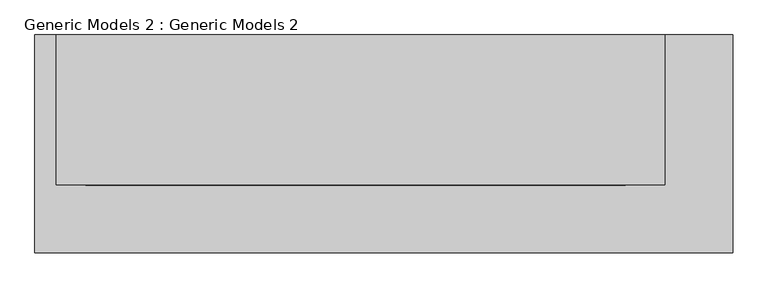
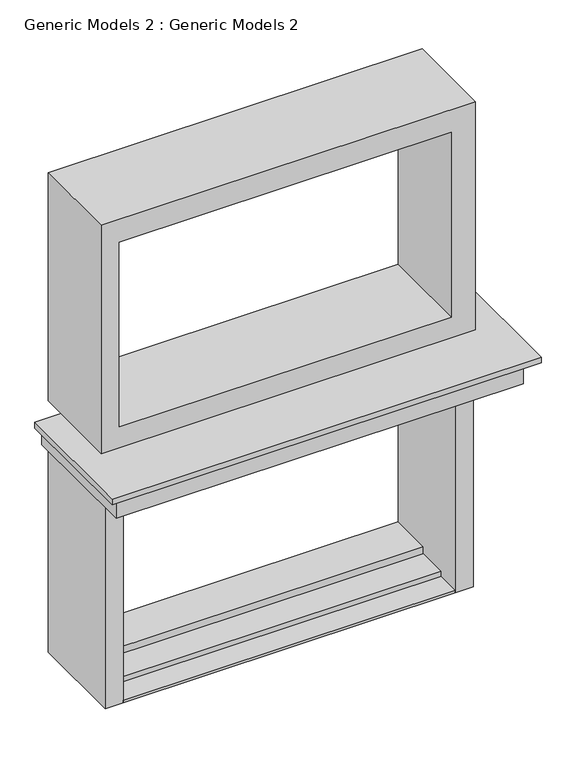
"""IFC4 building model written with IfcOpenShell, lengths in millimetres: proxy geometry, Generic Models 2 : Generic Models 2."""

from ifc_helpers import new_model, si_unit, frame, origin, origin_with_axes, place, context, project, spatial, polyline, outline, extrude, source, transform, mapped, element, save


def generic_models_2_generic_models_2_d251e182(model_context):
    return source(origin(), model_context, "Body", "SweptSolid", [
        extrude(outline(polyline([(3352.8, -18800.4761094), (3352.8, -14076.5127168), (6400.8, -14076.5127168), (6400.8, -18800.4761094), (3352.8, -18800.4761094)]), holes=[polyline([(3630.9088336, -18571.8761094), (6096.0, -18571.8761094), (6096.0, -14380.8761094), (3630.9088336, -14380.8761094), (3630.9088336, -18571.8761094)])]), frame((0.0, -16024.145609, 0.0), z_axis=(0.0, 1.0, 0.0), x_axis=(0.0, 0.0, 1.0)), (0.0, 0.0, 1.0), 1163.99946),
        extrude(outline(polyline([(-13549.4767283, -14860.146149), (-13549.4767283, -16547.7493682), (-18965.7783685, -16547.7493682), (-18965.7783685, -14860.146149), (-13549.4767283, -14860.146149)])), frame((0.0, 0.0, 3048.0), z_axis=(0.0, 0.0, 1.0), x_axis=(1.0, 0.0, 0.0)), (0.0, 0.0, 1.0), 76.2),
        extrude(outline(polyline([(-13733.3783685, -16482.1032767), (-18876.6761094, -16482.1032767), (-18876.6761094, -14860.146149), (-13733.3783685, -14860.146149), (-13733.3783685, -16482.1032767)])), frame((0.0, 0.0, 2794.612741), z_axis=(0.0, 0.0, 1.0), x_axis=(1.0, 0.0, 0.0)), (0.0, 0.0, 1.0), 253.387259),
        extrude(outline(polyline([(-18800.4761094, -16109.5913837), (-18800.4761094, -14860.146149), (-18571.8761094, -14860.146149), (-18571.8761094, -16109.5913837), (-18800.4761094, -16109.5913837)])), origin_with_axes(), (0.0, 0.0, 1.0), 2794.612741),
        extrude(outline(polyline([(-14152.2761094, -14860.146149), (-14152.2761094, -16109.5913837), (-14380.8761094, -16109.5913837), (-14380.8761094, -14860.146149), (-14152.2761094, -14860.146149)])), origin_with_axes(), (0.0, 0.0, 1.0), 2794.612741),
        extrude(outline(polyline([(-14380.8761094, -16109.5913837), (-18571.8761094, -16109.5913837), (-18571.8761094, -15804.7913837), (-14380.8761094, -15804.7913837), (-14380.8761094, -16109.5913837)])), origin_with_axes(), (0.0, 0.0, 1.0), 36.7484829),
        extrude(outline(polyline([(-14380.8761094, -15804.7913837), (-18571.8761094, -15804.7913837), (-18571.8761094, -15412.4825021), (-14380.8761094, -15412.4825021), (-14380.8761094, -15804.7913837)])), origin_with_axes(), (0.0, 0.0, 1.0), 102.2318862),
        extrude(outline(polyline([(-14380.8761094, -15412.4825021), (-18571.8761094, -15412.4825021), (-18571.8761094, -14860.146149), (-14380.8761094, -14860.146149), (-14380.8761094, -15412.4825021)])), origin_with_axes(), (0.0, 0.0, 1.0), 192.6917619),
    ])


if __name__ == "__main__":
    model = new_model("IFC4")
    model_context = context("Model", 3, world=origin())
    ifc_project = project(units=[si_unit("LENGTHUNIT", "METRE", prefix="MILLI")], contexts=[model_context])
    site = spatial("IfcSite", under=ifc_project)
    building = spatial("IfcBuilding", under=site)
    placement = place(None, origin())
    generic_models_2_generic_models_2_shape = generic_models_2_generic_models_2_d251e182(model_context)
    element("IfcBuildingElementProxy", 1, Name="Generic Models 2 : Generic Models 2", ObjectType="Generic Models 2 : Generic Models 2", at=placement, inside=building, context=model_context, shape_type="MappedRepresentation", body=[
        mapped(generic_models_2_generic_models_2_shape, transform((0.0, 0.0, 0.0), x_axis=(1.0, 0.0, 0.0), y_axis=(0.0, 1.0, 0.0), z_axis=(0.0, 0.0, 1.0))),
    ])
    save(model, "model.ifc")
